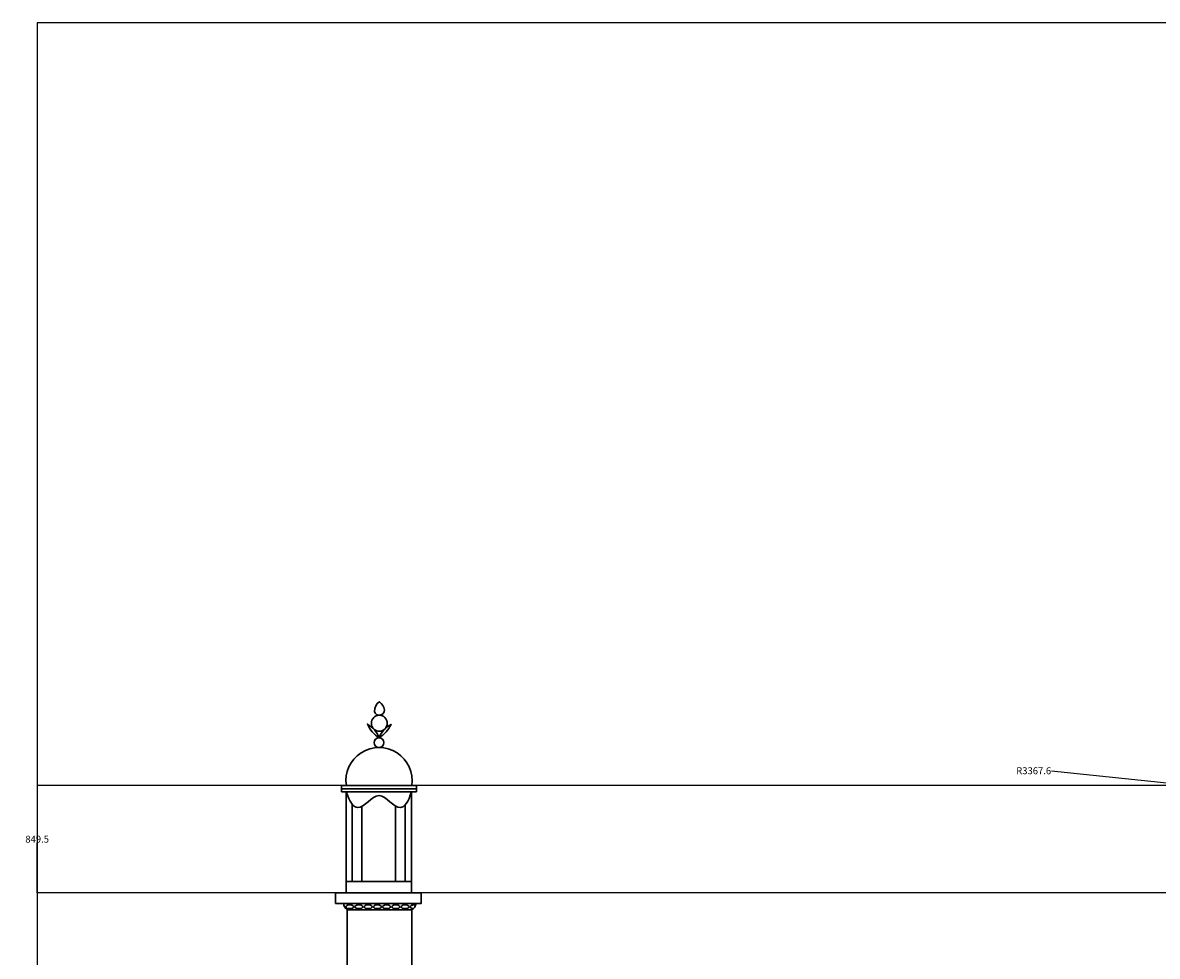
# Model space of a CAD drawing. Units: millimetres. Extents: x 8570 to 49085, y 3782 to 24863.
# Tile 3 of 15: x 8570 to 17549, y 17471 to 24863. Entities that reach past the tile are written whole.
import ezdxf

# ---------------------------------------------------------------- set-up
doc = ezdxf.new("R2010")
doc.units = ezdxf.units.MM
doc.header["$MEASUREMENT"] = 0
doc.header["$PDMODE"] = 3
doc.layers.add('A-ANNO-DIMS', color=2, linetype='Continuous', lineweight=18)
doc.layers.add('A-ELEV-MNRT', color=7, linetype='Continuous', lineweight=30)
doc.styles.get("Standard").update_dxf_attribs({"font": 'arial.ttf'})
doc.dimstyles.get("Standard").update_dxf_attribs({"dimtxt": 55, "dimasz": 0.18, "dimexe": 0.18, "dimexo": 0.0625, "dimgap": 0.09, "dimtad": 0, "dimtih": 1, "dimtoh": 1, "dimdec": 0, "dimzin": 0, "dimdsep": 46, "dimtxsty": 'Standard', "dimcen": 0.09, "dimadec": 0, "dimazin": 0, "dimtfac": 1, "dimtdec": 0, "dimtofl": 0, "dimtmove": 0, "dimatfit": 3, "dimfxl": 1, "dimtolj": 1, "dimtzin": 0, "dimarcsym": 0})

# ---------------------------------------------------------------- blocks, each defined once
blk = doc.blocks.new('MINARET-ELEV')
h = blk.add_hatch(color=256)
h.dxf.hatch_style = 1
edge = h.paths.add_edge_path()
edge.add_arc((788.1, 7879), 96, 347.52389, 357.31225, ccw=False)
edge.add_ellipse((859.2, 7847.7), major_axis=(31.8, 0), ratio=0.472441, start_angle=385.01443, end_angle=315.51296)
edge.add_arc((788.1, 7879), 96, 325.26025, 332.17741, ccw=False)
edge.add_line((867, 7824.3), (235, 7824.3))
edge.add_arc((313.9, 7879), 96, 182.68775, 214.73975, ccw=False)
edge.add_line((218, 7874.5), (884, 7874.5))
edge = h.paths.add_edge_path(flags=16)
edge.add_ellipse((494.2, 7847.7), major_axis=(31.8, 0), ratio=0.472441, start_angle=0, end_angle=360, ccw=False)
edge = h.paths.add_edge_path(flags=16)
edge.add_ellipse((567.2, 7847.7), major_axis=(31.8, 0), ratio=0.472441, start_angle=0, end_angle=360, ccw=False)
edge = h.paths.add_edge_path(flags=16)
edge.add_ellipse((421.2, 7847.7), major_axis=(31.8, 0), ratio=0.472441, start_angle=0, end_angle=360, ccw=False)
edge = h.paths.add_edge_path(flags=16)
edge.add_ellipse((640.2, 7847.7), major_axis=(31.8, 0), ratio=0.472441, start_angle=0, end_angle=360, ccw=False)
edge = h.paths.add_edge_path(flags=16)
edge.add_ellipse((348.2, 7847.7), major_axis=(31.8, 0), ratio=0.472441, start_angle=0, end_angle=360, ccw=False)
edge = h.paths.add_edge_path(flags=16)
edge.add_ellipse((713.2, 7847.7), major_axis=(31.8, 0), ratio=0.472441, start_angle=0, end_angle=360, ccw=False)
edge = h.paths.add_edge_path(flags=16)
edge.add_ellipse((275.2, 7847.7), major_axis=(31.8, 0), ratio=0.472441, start_angle=0, end_angle=360, ccw=False)
edge = h.paths.add_edge_path(flags=16)
edge.add_ellipse((786.2, 7847.7), major_axis=(31.8, 0), ratio=0.472441, start_angle=0, end_angle=360, ccw=False)
h = blk.add_hatch(color=256)
h.dxf.hatch_style = 1
edge = h.paths.add_edge_path()
edge.add_arc((940, 4615.3), 25, 270, 450, ccw=False)
edge.add_line((940, 4590.3), (160, 4590.3))
edge.add_arc((160, 4615.3), 25, 217.6761, 270, ccw=False)
edge.add_ellipse((127.2, 4613.7), major_axis=(31.8, 0), ratio=0.472441, start_angle=313.43175, end_angle=411.74889)
edge.add_arc((160, 4615.3), 25, 450, 510.08055, ccw=False)
edge.add_line((160, 4640.3), (940, 4640.3))
edge = h.paths.add_edge_path(flags=16)
edge.add_ellipse((347.2, 4613.7), major_axis=(31.8, 0), ratio=0.472441, start_angle=0, end_angle=360, ccw=False)
edge = h.paths.add_edge_path(flags=16)
edge.add_ellipse((420.2, 4613.7), major_axis=(31.8, 0), ratio=0.472441, start_angle=0, end_angle=360, ccw=False)
edge = h.paths.add_edge_path(flags=16)
edge.add_ellipse((274.2, 4613.7), major_axis=(31.8, 0), ratio=0.472441, start_angle=0, end_angle=360, ccw=False)
edge = h.paths.add_edge_path(flags=16)
edge.add_ellipse((493.2, 4613.7), major_axis=(31.8, 0), ratio=0.472441, start_angle=0, end_angle=360, ccw=False)
edge = h.paths.add_edge_path(flags=16)
edge.add_ellipse((198.8, 4613.7), major_axis=(31.8, 0), ratio=0.472441, start_angle=0, end_angle=360, ccw=False)
edge = h.paths.add_edge_path(flags=16)
edge.add_ellipse((566.2, 4613.7), major_axis=(31.8, 0), ratio=0.472441, start_angle=0, end_angle=360, ccw=False)
edge = h.paths.add_edge_path(flags=16)
edge.add_ellipse((639.2, 4613.7), major_axis=(31.8, 0), ratio=0.472441, start_angle=0, end_angle=360, ccw=False)
edge = h.paths.add_edge_path(flags=16)
edge.add_ellipse((712.2, 4613.7), major_axis=(31.8, 0), ratio=0.472441, start_angle=0, end_angle=360, ccw=False)
edge = h.paths.add_edge_path(flags=16)
edge.add_ellipse((785.2, 4613.7), major_axis=(31.8, 0), ratio=0.472441, start_angle=0, end_angle=360, ccw=False)
edge = h.paths.add_edge_path(flags=16)
edge.add_ellipse((858.2, 4613.7), major_axis=(31.8, 0), ratio=0.472441, start_angle=0, end_angle=360, ccw=False)
edge = h.paths.add_edge_path(flags=16)
edge.add_ellipse((931.2, 4613.7), major_axis=(31.8, 0), ratio=0.472441, start_angle=0, end_angle=360, ccw=False)
for p, q in [((851, 12922), (257.5, 12922)), ((257.5, 12922), (257.5, 12872)), ((851, 12897), (257.5, 12897)), ((851, 12872), (257.5, 12872)), ((298, 12162), (298, 12872)), ((556.7, 12843), (552, 12843)), ((815.5, 12162), (815.5, 12872)), ((851, 12922), (851, 12872)), ((348, 12162), (348, 12766.4)), ((423, 12162), (423, 12760.1)), ((690.5, 12162), (690.5, 12757.3)), ((765.5, 12162), (765.5, 12770.9)), ((815.5, 12162), (298, 12162)), ((807, 11939), (295, 11939)), ((867, 7824.3), (235, 7824.3)), ((867, 7824.3), (235, 7824.3)), ((160, 4590.3), (940, 4590.3)), ((165, 4590.3), (935, 4590.3)), ((905, 4590.3), (195, 4590.3)), ((300, 0), (300, 1321)), ((800, 0), (800, 1321)), ((1100, 0), (1100, 1321))]:
    blk.add_line(p, q)
blk.add_lwpolyline([(512, 13519.5, -0.216309), (551.3, 13585.8, -0.244698), (591, 13509.3, -0.244698)], format="xyb")
for points in [[(554, 13300, -0.140093), (458.9, 13405.9, -0.184272)], [(554, 13300, 0.140093), (646.7, 13408, 0.184272)]]:
    blk.add_lwpolyline(points, format="xyb", close=True)
for points in [[(815.5, 12072.5), (298, 12072.5), (298, 12162), (815.5, 12162)], [(898, 12072.5), (220.5, 12072.5), (220.5, 11989.2), (898, 11989.2)], [(948, 7939), (170.5, 7939), (170.5, 7874.5), (948, 7874.5)], [(997, 4705), (119.5, 4705), (119.5, 4640.5), (997, 4640.5)]]:
    blk.add_lwpolyline(points, close=True)
for points in [[(235, 7939), (235, 8939), (255, 8939), (255, 9939), (275, 9939), (275, 10939), (295, 10939), (295, 11939)], [(867, 7939), (867, 8939), (847, 8939), (847, 9939), (827, 9939), (827, 10939), (807, 10939), (807, 11939)], [(195, 4705), (195, 5705), (215, 5705), (215, 6705), (235, 6705), (235, 7824.3)], [(907, 4705), (907, 5705), (887, 5705), (887, 6705), (867, 6705), (867, 7824.3)], [(135, 1321), (135, 2321), (155, 2321), (155, 3321), (175, 3321), (175, 4321), (195, 4321), (195, 4590.3)], [(965, 1321), (965, 2321), (945, 2321), (945, 3321), (925, 3321), (925, 4321), (905, 4321), (905, 4590.3)], [(0, 1321), (1100, 1321)], [(0, 1246), (1100, 1246)]]:
    blk.add_lwpolyline(points)
for centre, radius in [((552, 13415.4), 63.1), ((554, 13261.5), 38.5)]:
    blk.add_circle(centre, radius)
for centre, radius, start, end in [((552, 13518.5), 40.1, 178.61203, 346.69346), ((554, 12961.3), 261.7, 351.36698, 188.63302), ((330.8, 12000.6), 71.3, 189.21146, 239.80255), ((759.2, 12000.8), 78.1, 307.68318, 351.42034), ((313.9, 7879), 96, 182.68775, 214.73975), ((788.1, 7879), 96, 325.26025, 357.31225), ((160, 4615.3), 25, 90, 270), ((940, 4615.3), 25, 270, 90)]:
    blk.add_arc(centre, radius, start, end)
at = {"extrusion": (0, 0, -1)}
for centre, start_param, end_param in [((275.2, 11962.4), -1.939365, 1.327018), ((348.2, 11962.4), -6.283185, 0), ((421.2, 11962.4), -6.283185, 0), ((494.2, 11962.4), -6.283185, 0), ((567.2, 11962.4), -6.283185, 0), ((640.2, 11962.4), -6.283185, 0), ((713.2, 11962.4), -6.283185, 0), ((786.2, 11962.4), -6.283185, 0), ((275.2, 7847.7), -6.283185, 0), ((348.2, 7847.7), -6.283185, 0), ((421.2, 7847.7), -6.283185, 0), ((494.2, 7847.7), -6.283185, 0), ((567.2, 7847.7), -6.283185, 0), ((640.2, 7847.7), -6.283185, 0), ((713.2, 7847.7), -6.283185, 0), ((786.2, 7847.7), -6.283185, 0), ((859.2, 7847.7), -5.160703, -0.779193), ((127.2, 4613.7), -1.214257, 1.150222), ((198.8, 4613.7), -6.283185, 0), ((274.2, 4613.7), -6.283185, 0), ((347.2, 4613.7), -6.283185, 0), ((420.2, 4613.7), -6.283185, 0), ((493.2, 4613.7), -6.283185, 0), ((566.2, 4613.7), -6.283185, 0), ((639.2, 4613.7), -6.283185, 0), ((712.2, 4613.7), -6.283185, 0), ((785.2, 4613.7), -6.283185, 0), ((858.2, 4613.7), -6.283185, 0), ((931.2, 4613.7), -6.283185, 0)]:
    blk.add_ellipse(centre, major_axis=(31.8, 0), ratio=0.472441, start_param=start_param, end_param=end_param, dxfattribs=at)
for points in [[(554.4, 12843), (553.6, 12843), (500.8, 12843), (391.9, 12680.1), (321.9, 12795.7), (298, 12872)], [(554.4, 12843), (555.2, 12843), (607.9, 12843), (716.8, 12680.1), (786.9, 12795.7), (815.5, 12872)]]:
    blk.add_open_spline(points, degree=3, knots=[136.061972, 136.061972, 136.061972, 136.061972, 139.000899, 330.944902, 463.724089, 463.724089, 463.724089, 463.724089])
blk = doc.blocks.new('*D44')
at = {"layer": 'A-ANNO-DIMS', "color": 0, "lineweight": -2, "transparency": 16777216}
for p, q in [((22399.7, 24863), (8684.3, 24863)), ((8684.5, 24862.8), (8684.5, 15410.4)), ((8684.5, 5901.7), (8684.5, 15354.1)), ((10843.9, 5901.5), (8684.3, 5901.5))]:
    blk.add_line(p, q, dxfattribs=at)
at = {"layer": 'A-ANNO-DIMS', "color": 0, "transparency": 16777216}
for points in [[(8684.5, 24862.8), (8684.5, 24862.8), (8684.5, 24863)], [(8684.5, 5901.7), (8684.5, 5901.7), (8684.5, 5901.5)]]:
    blk.add_solid(points, dxfattribs=at)
at = {"layer": 'Defpoints', "color": 0, "transparency": 16777216}
for p in [(8684.5, 24863), (22399.8, 24863), (10844, 5901.5)]:
    blk.add_point(p, dxfattribs=at)
at = {"layer": 'A-ANNO-DIMS', "color": 0, "transparency": 16777216, "insert": (8684.5, 15382.2), "char_height": 55, "attachment_point": 5}
blk.add_mtext('\\A1;18961', dxfattribs=at)
blk = doc.blocks.new('*D61')
at = {"layer": 'A-ANNO-DIMS', "color": 0, "lineweight": -2, "transparency": 16777216}
for p, q in [((33091.4, 17974), (8684.3, 17974)), ((8684.5, 17973.8), (8684.5, 15935.4)), ((8684.5, 13840.7), (8684.5, 15879.1)), ((33041.4, 13840.5), (8684.3, 13840.5))]:
    blk.add_line(p, q, dxfattribs=at)
at = {"layer": 'A-ANNO-DIMS', "color": 0, "transparency": 16777216}
for points in [[(8684.5, 17973.8), (8684.5, 17973.8), (8684.5, 17974)], [(8684.5, 13840.7), (8684.5, 13840.7), (8684.5, 13840.5)]]:
    blk.add_solid(points, dxfattribs=at)
at = {"layer": 'Defpoints', "color": 0, "transparency": 16777216}
for p in [(8684.5, 17974), (33091.5, 17974), (33041.5, 13840.5)]:
    blk.add_point(p, dxfattribs=at)
at = {"layer": 'A-ANNO-DIMS', "color": 0, "transparency": 16777216, "insert": (8684.5, 15907.2), "char_height": 55, "attachment_point": 5}
blk.add_mtext('\\A1;4133.5', dxfattribs=at)
blk = doc.blocks.new('*D62')
at = {"layer": 'A-ANNO-DIMS', "color": 0, "lineweight": -2, "transparency": 16777216}
for p, q in [((33128.4, 18823.5), (8684.3, 18823.5)), ((8684.5, 18823.3), (8684.5, 18426.9)), ((8684.5, 17974.2), (8684.5, 18370.6)), ((33091.4, 17974), (8684.3, 17974))]:
    blk.add_line(p, q, dxfattribs=at)
at = {"layer": 'A-ANNO-DIMS', "color": 0, "transparency": 16777216}
for points in [[(8684.5, 18823.3), (8684.5, 18823.3), (8684.5, 18823.5)], [(8684.5, 17974.2), (8684.5, 17974.2), (8684.5, 17974)]]:
    blk.add_solid(points, dxfattribs=at)
at = {"layer": 'Defpoints', "color": 0, "transparency": 16777216}
for p in [(8684.5, 18823.5), (33128.5, 18823.5), (33091.5, 17974)]:
    blk.add_point(p, dxfattribs=at)
at = {"layer": 'A-ANNO-DIMS', "color": 0, "transparency": 16777216, "insert": (8684.5, 18398.7), "char_height": 55, "attachment_point": 5}
blk.add_mtext('\\A1;849.5', dxfattribs=at)
blk = doc.blocks.new('*D79')
at = {"layer": 'A-ANNO-DIMS', "color": 0, "lineweight": -2, "transparency": 16777216}
for p, q in [((16711.1, 18940.6), (18720.6, 18730.8)), ((22070.1, 18381.1), (22070.3, 18381.1)), ((22070.2, 18381), (22070.2, 18381.1))]:
    blk.add_line(p, q, dxfattribs=at)
at = {"layer": 'A-ANNO-DIMS', "color": 0, "transparency": 16777216}
blk.add_solid([(18720.6, 18730.8), (18720.6, 18730.7), (18720.7, 18730.8)], dxfattribs=at)
at = {"layer": 'Defpoints', "color": 0, "transparency": 16777216}
for p in [(18720.7, 18730.8), (22070.2, 18381.1)]:
    blk.add_point(p, dxfattribs=at)
at = {"layer": 'A-ANNO-DIMS', "color": 0, "transparency": 16777216, "insert": (16570.5, 18940.6), "char_height": 55, "attachment_point": 5}
blk.add_mtext('\\A1;R3367.6', dxfattribs=at)

msp = doc.modelspace()

# ---------------------------------------------------------------- block references
at = {"layer": 'A-ELEV-MNRT', "extrusion": (0, 0, -1), "zscale": -1}
msp.add_blockref('MINARET-ELEV', (-11944, 5901.5), dxfattribs=at)

# ---------------------------------------------------------------- dimensions: what is measured, and where the dimension line sits
at = {"layer": 'A-ANNO-DIMS'}
for base, p1, p2, override, picture, middle in [((8684.5, 24862.95), (10844, 5901.5), (22399.75, 24862.95), {"dimdec": 0, "dimlfac": 1, "dimrnd": 0, "dimzin": 0, "dimdsep": 46, "dimlunit": 2}, '*D44', (8684.5, 15382.23)), ((8684.5, 18823.5), (33091.5, 17974), (33128.5, 18823.5), {"dimdec": 1, "dimlfac": 1, "dimrnd": 0, "dimzin": 0, "dimdsep": 46, "dimlunit": 2}, '*D62', (8684.5, 18398.75)), ((8684.5, 17974), (33041.5, 13840.5), (33091.5, 17974), {"dimdec": 1, "dimlfac": 1, "dimrnd": 0, "dimzin": 0, "dimdsep": 46, "dimlunit": 2}, '*D61', (8684.5, 15907.25))]:
    dim = msp.add_linear_dim(base=base, p1=p1, p2=p2, angle=90, dimstyle='Standard', override=override, dxfattribs=at)
    dim.commit()
    dim.dimension.update_dxf_attribs({"geometry": picture, "text_midpoint": middle})
dim = msp.add_radius_dim(center=(22070.17, 18381.06), mpoint=(18720.74, 18730.75), dimstyle='Standard', override={"dimdec": 1, "dimlfac": 1, "dimrnd": 0, "dimzin": 0, "dimdsep": 46, "dimlunit": 2}, dxfattribs=at)
dim.commit()
dim.dimension.update_dxf_attribs({"geometry": '*D79', "text_midpoint": (16711.08, 18940.57), "dimtype": 164})

doc.saveas('drawing.dxf')
